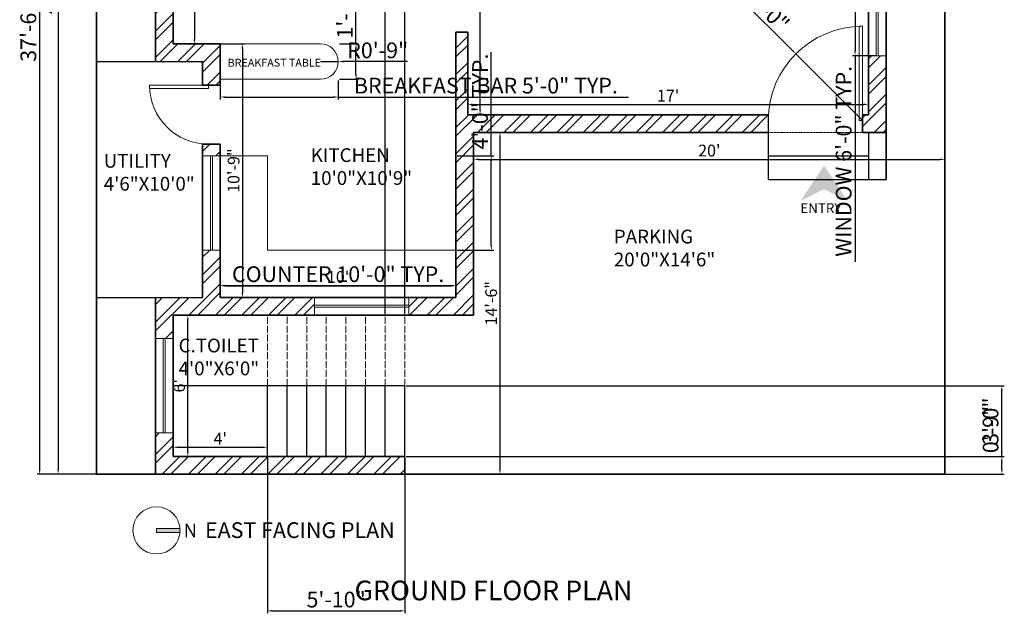
# Model space of a CAD drawing. Units: inches. Extents: x 4732 to 5926, y 2665 to 3255.
# Tile 7 of 8: x 5425 to 5926, y 2665 to 2967. Entities that reach past the tile are written whole.
import ezdxf

# ---------------------------------------------------------------- set-up
doc = ezdxf.new("R2010")
doc.units = ezdxf.units.IN
doc.linetypes.add('ACAD_ISO02W100', pattern=[15, 12, -3])
for name, color, linetype, lineweight in [('A-ANNO-DIMS', 2, 'Continuous', 18), ('A-ANNO-SYMB', 7, 'Continuous', 18), ('A-ANNO-TEXT', 7, 'Continuous', 18), ('A-ANNO-TITL', 7, 'Continuous', 25), ('A-AREA-IDEN', 7, 'Continuous', 18), ('A-DOOR', 3, 'Continuous', 18), ('A-FLOR', 7, 'Continuous', 25), ('A-FLOR-CASE', 7, 'Continuous', 18), ('A-FLOR-STRS', 7, 'Continuous', 25), ('A-FLOR-STRS-HIDN', 8, 'ACAD_ISO02W100', 18), ('A-GLAZ', 4, 'Continuous', 18), ('A-WALL', 7, 'Continuous', 35), ('A-WALL-PATT', 8, 'Continuous', 13), ('C-PROP', 7, 'Continuous', 35)]:
    doc.layers.add(name, color=color, linetype=linetype, lineweight=lineweight)
doc.styles.get("Standard").update_dxf_attribs({"font": 'arial.ttf'})
doc.dimstyles.new('ISO-25', dxfattribs={"dimtxt": 8, "dimasz": 2.5, "dimexe": 1.25, "dimexo": 0.625, "dimtad": 1, "dimdec": 1, "dimlunit": 3, "dimtxsty": 'Standard', "dimcen": 2.5, "dimadec": 0, "dimazin": 0, "dimtfac": 1, "dimtdec": 1, "dimtmove": 0, "dimatfit": 3, "dimfxl": 1, "dimarcsym": 0})

# ---------------------------------------------------------------- blocks, each defined once
blk = doc.blocks.new('*U19')
for p, q in [((0, 0), (0, -6)), ((30, 0), (30, -6))]:
    blk.add_line(p, q)
blk.add_lwpolyline([(0, 0), (0, 30), (1.75, 30), (1.75, 0)], close=True)
blk.add_arc((0, 0), 30, 0, 90)
blk = doc.blocks.new('*D30')
at = {"layer": 'A-ANNO-DIMS', "color": 0, "lineweight": -2, "transparency": 16777216}
for p, q in [((5463.31, 3215.93), (5443.14, 3215.93)), ((5444.39, 3213.43), (5444.39, 2738.43)), ((5463.31, 2735.93), (5443.14, 2735.93))]:
    blk.add_line(p, q, dxfattribs=at)
at = {"layer": 'A-ANNO-DIMS', "color": 0, "transparency": 16777216}
for points in [[(5443.98, 3213.43), (5444.81, 3213.43), (5444.39, 3215.93)], [(5443.98, 2738.43), (5444.81, 2738.43), (5444.39, 2735.93)]]:
    blk.add_solid(points, dxfattribs=at)
at = {"layer": 'Defpoints', "color": 0, "transparency": 16777216}
for p in [(5463.94, 3215.93), (5444.39, 2735.93), (5463.94, 2735.93)]:
    blk.add_point(p, dxfattribs=at)
at = {"layer": 'A-ANNO-DIMS', "color": 0, "transparency": 16777216, "insert": (5440.71, 2975.93), "char_height": 6, "attachment_point": 5, "rotation": 90}
blk.add_mtext("40'", dxfattribs=at)
blk = doc.blocks.new('*D31')
at = {"layer": 'A-ANNO-DIMS', "color": 0, "lineweight": -2, "transparency": 16777216}
for p, q in [((5502.94, 2750.26), (5502.94, 2750.89)), ((5505.44, 2749.64), (5548.44, 2749.64)), ((5550.94, 2750.26), (5550.94, 2750.89))]:
    blk.add_line(p, q, dxfattribs=at)
at = {"layer": 'A-ANNO-DIMS', "color": 0, "transparency": 16777216}
for points in [[(5505.44, 2750.05), (5505.44, 2749.22), (5502.94, 2749.64)], [(5548.44, 2750.05), (5548.44, 2749.22), (5550.94, 2749.64)]]:
    blk.add_solid(points, dxfattribs=at)
at = {"layer": 'Defpoints', "color": 0, "transparency": 16777216}
for p in [(5502.94, 2749.64), (5550.94, 2749.64), (5550.94, 2749.64)]:
    blk.add_point(p, dxfattribs=at)
at = {"layer": 'A-ANNO-DIMS', "color": 0, "transparency": 16777216, "insert": (5526.94, 2753.26), "char_height": 6, "attachment_point": 5}
blk.add_mtext("4'", dxfattribs=at)
blk = doc.blocks.new('*D32')
at = {"layer": 'A-ANNO-DIMS', "color": 0, "lineweight": -2, "transparency": 16777216}
for p, q in [((5503.56, 2816.93), (5511.66, 2816.93)), ((5510.41, 2747.43), (5510.41, 2814.43)), ((5503.56, 2744.93), (5511.66, 2744.93))]:
    blk.add_line(p, q, dxfattribs=at)
at = {"layer": 'A-ANNO-DIMS', "color": 0, "transparency": 16777216}
for points in [[(5510, 2814.43), (5510.83, 2814.43), (5510.41, 2816.93)], [(5510, 2747.43), (5510.83, 2747.43), (5510.41, 2744.93)]]:
    blk.add_solid(points, dxfattribs=at)
at = {"layer": 'Defpoints', "color": 0, "transparency": 16777216}
for p in [(5502.94, 2816.93), (5510.41, 2816.93), (5502.94, 2744.93)]:
    blk.add_point(p, dxfattribs=at)
at = {"layer": 'A-ANNO-DIMS', "color": 0, "transparency": 16777216, "insert": (5506.72, 2780.93), "char_height": 6, "attachment_point": 5, "rotation": 90}
blk.add_mtext("6'", dxfattribs=at)
blk = doc.blocks.new('*D33')
at = {"layer": 'A-ANNO-DIMS', "color": 0, "lineweight": -2, "transparency": 16777216}
for p, q in [((5526.94, 2826.56), (5526.94, 2833.08)), ((5646.94, 2826.56), (5646.94, 2833.08)), ((5529.44, 2831.83), (5644.44, 2831.83))]:
    blk.add_line(p, q, dxfattribs=at)
at = {"layer": 'A-ANNO-DIMS', "color": 0, "transparency": 16777216}
for points in [[(5529.44, 2832.25), (5529.44, 2831.42), (5526.94, 2831.83)], [(5644.44, 2832.25), (5644.44, 2831.42), (5646.94, 2831.83)]]:
    blk.add_solid(points, dxfattribs=at)
at = {"layer": 'Defpoints', "color": 0, "transparency": 16777216}
for p in [(5646.94, 2831.83), (5526.94, 2825.93), (5646.94, 2825.93)]:
    blk.add_point(p, dxfattribs=at)
at = {"layer": 'A-ANNO-DIMS', "color": 0, "transparency": 16777216, "insert": (5586.94, 2835.52), "char_height": 6, "attachment_point": 5}
blk.add_mtext("10'", dxfattribs=at)
blk = doc.blocks.new('*D34')
at = {"layer": 'A-ANNO-DIMS', "color": 0, "lineweight": -2, "transparency": 16777216}
for p, q in [((5518.56, 2954.93), (5539.45, 2954.93)), ((5538.2, 2952.43), (5538.2, 2828.43)), ((5527.56, 2825.93), (5539.45, 2825.93))]:
    blk.add_line(p, q, dxfattribs=at)
at = {"layer": 'A-ANNO-DIMS', "color": 0, "transparency": 16777216}
for points in [[(5537.78, 2952.43), (5538.61, 2952.43), (5538.2, 2954.93)], [(5537.78, 2828.43), (5538.61, 2828.43), (5538.2, 2825.93)]]:
    blk.add_solid(points, dxfattribs=at)
at = {"layer": 'Defpoints', "color": 0, "transparency": 16777216}
for p in [(5517.94, 2954.93), (5526.94, 2825.93), (5538.2, 2825.93)]:
    blk.add_point(p, dxfattribs=at)
at = {"layer": 'A-ANNO-DIMS', "color": 0, "transparency": 16777216, "insert": (5534.51, 2890.43), "char_height": 6, "attachment_point": 5, "rotation": 90}
blk.add_mtext('10\'-9"', dxfattribs=at)
blk = doc.blocks.new('*D35')
at = {"layer": 'A-ANNO-DIMS', "color": 0, "lineweight": -2, "transparency": 16777216}
for p, q in [((5503.56, 3050.93), (5515.02, 3050.93)), ((5513.77, 3048.43), (5513.77, 2957.43)), ((5503.56, 2954.93), (5515.02, 2954.93))]:
    blk.add_line(p, q, dxfattribs=at)
at = {"layer": 'A-ANNO-DIMS', "color": 0, "transparency": 16777216}
for points in [[(5513.36, 3048.43), (5514.19, 3048.43), (5513.77, 3050.93)], [(5513.36, 2957.43), (5514.19, 2957.43), (5513.77, 2954.93)]]:
    blk.add_solid(points, dxfattribs=at)
at = {"layer": 'Defpoints', "color": 0, "transparency": 16777216}
for p in [(5502.94, 3050.93), (5502.94, 2954.93), (5513.77, 2954.93)]:
    blk.add_point(p, dxfattribs=at)
at = {"layer": 'A-ANNO-DIMS', "color": 0, "transparency": 16777216, "insert": (5510.08, 3002.93), "char_height": 6, "attachment_point": 5, "rotation": 90}
blk.add_mtext("8'", dxfattribs=at)
blk = doc.blocks.new('*D37')
at = {"layer": 'A-ANNO-DIMS', "color": 0, "lineweight": -2, "transparency": 16777216}
for p, q in [((5652.94, 2919.56), (5652.94, 2925.42)), ((5655.44, 2924.17), (5854.44, 2924.17)), ((5856.94, 2919.56), (5856.94, 2925.42))]:
    blk.add_line(p, q, dxfattribs=at)
at = {"layer": 'A-ANNO-DIMS', "color": 0, "transparency": 16777216}
for points in [[(5655.44, 2924.59), (5655.44, 2923.75), (5652.94, 2924.17)], [(5854.44, 2924.59), (5854.44, 2923.75), (5856.94, 2924.17)]]:
    blk.add_solid(points, dxfattribs=at)
at = {"layer": 'Defpoints', "color": 0, "transparency": 16777216}
for p in [(5856.94, 2924.17), (5652.94, 2918.93), (5856.94, 2918.93)]:
    blk.add_point(p, dxfattribs=at)
at = {"layer": 'A-ANNO-DIMS', "color": 0, "transparency": 16777216, "insert": (5754.94, 2927.81), "char_height": 6, "attachment_point": 5}
blk.add_mtext("17'", dxfattribs=at)
blk = doc.blocks.new('*D38')
at = {"layer": 'A-ANNO-DIMS', "color": 0, "lineweight": -2, "transparency": 16777216}
for p, q in [((5653.56, 3050.93), (5660.5, 3050.93)), ((5659.25, 2921.43), (5659.25, 3048.43)), ((5653.56, 2918.93), (5660.5, 2918.93))]:
    blk.add_line(p, q, dxfattribs=at)
at = {"layer": 'A-ANNO-DIMS', "color": 0, "transparency": 16777216}
for points in [[(5658.83, 3048.43), (5659.67, 3048.43), (5659.25, 3050.93)], [(5658.83, 2921.43), (5659.67, 2921.43), (5659.25, 2918.93)]]:
    blk.add_solid(points, dxfattribs=at)
at = {"layer": 'Defpoints', "color": 0, "transparency": 16777216}
for p in [(5652.94, 3050.93), (5659.25, 3050.93), (5652.94, 2918.93)]:
    blk.add_point(p, dxfattribs=at)
at = {"layer": 'A-ANNO-DIMS', "color": 0, "transparency": 16777216, "insert": (5655.61, 2984.93), "char_height": 6, "attachment_point": 5, "rotation": 90}
blk.add_mtext("11'", dxfattribs=at)
blk = doc.blocks.new('*D52')
at = {"layer": 'A-ANNO-DIMS', "color": 0, "lineweight": -2, "transparency": 16777216}
for p, q in [((5655.94, 2909.31), (5655.94, 2894.94)), ((5895.94, 2909.31), (5895.94, 2894.94)), ((5658.44, 2896.19), (5893.44, 2896.19))]:
    blk.add_line(p, q, dxfattribs=at)
at = {"layer": 'A-ANNO-DIMS', "color": 0, "transparency": 16777216}
for points in [[(5658.44, 2896.61), (5658.44, 2895.78), (5655.94, 2896.19)], [(5893.44, 2896.61), (5893.44, 2895.78), (5895.94, 2896.19)]]:
    blk.add_solid(points, dxfattribs=at)
at = {"layer": 'Defpoints', "color": 0, "transparency": 16777216}
for p in [(5655.94, 2909.93), (5895.94, 2909.93), (5895.94, 2896.19)]:
    blk.add_point(p, dxfattribs=at)
at = {"layer": 'A-ANNO-DIMS', "color": 0, "transparency": 16777216, "insert": (5775.94, 2899.88), "char_height": 6, "attachment_point": 5}
blk.add_mtext("20'", dxfattribs=at)
blk = doc.blocks.new('*D53')
at = {"layer": 'A-ANNO-DIMS', "color": 0, "lineweight": -2, "transparency": 16777216}
for p, q in [((5656.56, 2909.93), (5670.58, 2909.93)), ((5669.33, 2907.43), (5669.33, 2738.43)), ((5656.56, 2735.93), (5670.58, 2735.93))]:
    blk.add_line(p, q, dxfattribs=at)
at = {"layer": 'A-ANNO-DIMS', "color": 0, "transparency": 16777216}
for points in [[(5668.92, 2907.43), (5669.75, 2907.43), (5669.33, 2909.93)], [(5668.92, 2738.43), (5669.75, 2738.43), (5669.33, 2735.93)]]:
    blk.add_solid(points, dxfattribs=at)
at = {"layer": 'Defpoints', "color": 0, "transparency": 16777216}
for p in [(5655.94, 2909.93), (5655.94, 2735.93), (5669.33, 2735.93)]:
    blk.add_point(p, dxfattribs=at)
at = {"layer": 'A-ANNO-DIMS', "color": 0, "transparency": 16777216, "insert": (5665.64, 2822.93), "char_height": 6, "attachment_point": 5, "rotation": 90}
blk.add_mtext('14\'-6"', dxfattribs=at)
blk = doc.blocks.new('GLAZ-UNIT-48IN')
for p, q in [((0, 1), (48, 1)), ((0, 0), (48, 0))]:
    blk.add_line(p, q)
blk = doc.blocks.new('GLAZ-UNIT-72IN')
for p, q in [((0, 72), (0, 0)), ((1, 72), (1, 0))]:
    blk.add_line(p, q)
blk = doc.blocks.new('COUNTER-KITCHEN-L')
for p, q in [((0, 48), (24, 48)), ((24, 0), (24, 48)), ((24, 0), (120, 0))]:
    blk.add_line(p, q)
blk = doc.blocks.new('COUNTER-BREAKFAST')
for p, q in [((0, 18), (51.1, 18)), ((0, 0), (51.1, 0))]:
    blk.add_line(p, q)
blk.add_arc((51.1, 9), 9, 270, 90)
blk = doc.blocks.new('NORTH-INDICATOR')
at = {"transparency": 33554687}
h = blk.add_hatch(color=256, dxfattribs=at)
h.dxf.hatch_style = 1
h.paths.add_polyline_path([(0, 1), (0, -1), (11.96, -1, 0.020861), (12, 0, 0.020861), (11.96, 1)])
for p, q in [((0, -1), (0, 1)), ((0, 1), (11.96, 1)), ((12, -1), (0, -1))]:
    blk.add_line(p, q)
blk.add_circle((0, 0), 12)
blk.add_text('N', height=6.9).set_placement((13.83, -3.53))
blk = doc.blocks.new('*D68')
at = {"layer": 'A-ANNO-DIMS', "color": 0, "lineweight": -2, "transparency": 16777216}
for p, q in [((5860.31, 3020.93), (5848.89, 3020.93)), ((5850.14, 3018.43), (5850.14, 2951.43)), ((5860.31, 2948.93), (5848.89, 2948.93)), ((5850.14, 2948.93), (5850.14, 2843.95))]:
    blk.add_line(p, q, dxfattribs=at)
at = {"layer": 'A-ANNO-DIMS', "color": 0, "transparency": 16777216}
for points in [[(5849.72, 3018.43), (5850.55, 3018.43), (5850.14, 3020.93)], [(5849.72, 2951.43), (5850.55, 2951.43), (5850.14, 2948.93)]]:
    blk.add_solid(points, dxfattribs=at)
at = {"layer": 'Defpoints', "color": 0, "transparency": 16777216}
for p in [(5860.94, 3020.93), (5850.14, 2948.93), (5860.94, 2948.93)]:
    blk.add_point(p, dxfattribs=at)
at = {"layer": 'A-ANNO-DIMS', "color": 0, "transparency": 16777216, "insert": (5845.37, 2895.19), "char_height": 8, "attachment_point": 5, "rotation": 90}
blk.add_mtext('WINDOW 6\'-0" TYP.', dxfattribs=at)
blk = doc.blocks.new('*D70')
at = {"layer": 'A-ANNO-DIMS', "color": 0, "lineweight": -2, "transparency": 16777216}
for p, q in [((5526.94, 2849.31), (5526.94, 2830.68)), ((5646.94, 2849.31), (5646.94, 2830.68)), ((5529.44, 2831.93), (5644.44, 2831.93))]:
    blk.add_line(p, q, dxfattribs=at)
at = {"layer": 'A-ANNO-DIMS', "color": 0, "transparency": 16777216}
for points in [[(5529.44, 2832.35), (5529.44, 2831.52), (5526.94, 2831.93)], [(5644.44, 2832.35), (5644.44, 2831.52), (5646.94, 2831.93)]]:
    blk.add_solid(points, dxfattribs=at)
at = {"layer": 'Defpoints', "color": 0, "transparency": 16777216}
for p in [(5526.94, 2849.93), (5646.94, 2849.93), (5646.94, 2831.93)]:
    blk.add_point(p, dxfattribs=at)
at = {"layer": 'A-ANNO-DIMS', "color": 0, "transparency": 16777216, "insert": (5586.94, 2836.7), "char_height": 8, "attachment_point": 5}
blk.add_mtext('COUNTER 10\'-0" TYP.', dxfattribs=at)
blk = doc.blocks.new('*D71')
at = {"layer": 'A-ANNO-DIMS', "color": 0, "lineweight": -2, "transparency": 16777216}
for p, q in [((5664.94, 2897.93), (5664.94, 2950.77)), ((5647.56, 2897.93), (5666.19, 2897.93)), ((5664.94, 2852.43), (5664.94, 2895.43)), ((5647.56, 2849.93), (5666.19, 2849.93))]:
    blk.add_line(p, q, dxfattribs=at)
at = {"layer": 'A-ANNO-DIMS', "color": 0, "transparency": 16777216}
for points in [[(5664.52, 2895.43), (5665.35, 2895.43), (5664.94, 2897.93)], [(5664.52, 2852.43), (5665.35, 2852.43), (5664.94, 2849.93)]]:
    blk.add_solid(points, dxfattribs=at)
at = {"layer": 'Defpoints', "color": 0, "transparency": 16777216}
for p in [(5646.94, 2897.93), (5664.94, 2897.93), (5646.94, 2849.93)]:
    blk.add_point(p, dxfattribs=at)
at = {"layer": 'A-ANNO-DIMS', "color": 0, "transparency": 16777216, "insert": (5660.23, 2925.6), "char_height": 8, "attachment_point": 5, "rotation": 90}
blk.add_mtext('4\'-0" TYP.', dxfattribs=at)
blk = doc.blocks.new('*D72')
at = {"layer": 'A-ANNO-DIMS', "color": 0, "lineweight": -2, "transparency": 16777216}
for p, q in [((5526.94, 2936.31), (5526.94, 2926.67)), ((5587.04, 2936.31), (5587.04, 2926.67)), ((5529.44, 2927.92), (5584.54, 2927.92)), ((5587.04, 2927.92), (5734.84, 2927.92))]:
    blk.add_line(p, q, dxfattribs=at)
at = {"layer": 'A-ANNO-DIMS', "color": 0, "transparency": 16777216}
for points in [[(5529.44, 2928.33), (5529.44, 2927.5), (5526.94, 2927.92)], [(5584.54, 2928.33), (5584.54, 2927.5), (5587.04, 2927.92)]]:
    blk.add_solid(points, dxfattribs=at)
at = {"layer": 'Defpoints', "color": 0, "transparency": 16777216}
for p in [(5526.94, 2936.93), (5587.04, 2936.93), (5587.04, 2927.92)]:
    blk.add_point(p, dxfattribs=at)
at = {"layer": 'A-ANNO-DIMS', "color": 0, "transparency": 16777216, "insert": (5662.19, 2932.68), "char_height": 8, "attachment_point": 5}
blk.add_mtext('BREAKFAST BAR 5\'-0" TYP.', dxfattribs=at)
blk = doc.blocks.new('*D73')
at = {"layer": 'A-ANNO-DIMS', "color": 0, "lineweight": -2, "transparency": 16777216}
for p, q in [((5596.05, 2954.93), (5596.05, 3006.69)), ((5587.66, 2954.93), (5597.3, 2954.93)), ((5596.05, 2939.43), (5596.05, 2952.43)), ((5587.66, 2936.93), (5597.3, 2936.93))]:
    blk.add_line(p, q, dxfattribs=at)
at = {"layer": 'A-ANNO-DIMS', "color": 0, "transparency": 16777216}
for points in [[(5595.64, 2952.43), (5596.47, 2952.43), (5596.05, 2954.93)], [(5595.64, 2939.43), (5596.47, 2939.43), (5596.05, 2936.93)]]:
    blk.add_solid(points, dxfattribs=at)
at = {"layer": 'Defpoints', "color": 0, "transparency": 16777216}
for p in [(5587.04, 2954.93), (5596.05, 2954.93), (5587.04, 2936.93)]:
    blk.add_point(p, dxfattribs=at)
at = {"layer": 'A-ANNO-DIMS', "color": 0, "transparency": 16777216, "insert": (5591.34, 2982.06), "char_height": 8, "attachment_point": 5, "rotation": 90}
blk.add_mtext('1\'-6" TYP.', dxfattribs=at)
blk = doc.blocks.new('*D105')
at = {"layer": 'A-ANNO-DIMS', "color": 0, "lineweight": -2, "transparency": 16777216}
for p, q in [((5493.31, 3185.93), (5433.74, 3185.93)), ((5434.99, 3183.43), (5434.99, 2738.43)), ((5493.31, 2735.93), (5433.74, 2735.93))]:
    blk.add_line(p, q, dxfattribs=at)
at = {"layer": 'A-ANNO-DIMS', "color": 0, "transparency": 16777216}
for points in [[(5434.57, 3183.43), (5435.4, 3183.43), (5434.99, 3185.93)], [(5434.57, 2738.43), (5435.4, 2738.43), (5434.99, 2735.93)]]:
    blk.add_solid(points, dxfattribs=at)
at = {"layer": 'Defpoints', "color": 0, "transparency": 16777216}
for p in [(5493.94, 3185.93), (5434.99, 2735.93), (5493.94, 2735.93)]:
    blk.add_point(p, dxfattribs=at)
at = {"layer": 'A-ANNO-DIMS', "color": 0, "transparency": 16777216, "insert": (5430.27, 2960.93), "char_height": 8, "attachment_point": 5, "rotation": 90}
blk.add_mtext('37\'-6"', dxfattribs=at)
blk = doc.blocks.new('*D110')
at = {"layer": 'A-ANNO-DIMS', "color": 0, "lineweight": -2, "transparency": 16777216}
for p, q in [((5550.94, 2744.31), (5550.94, 2665.12)), ((5620.94, 2744.31), (5620.94, 2665.12)), ((5553.44, 2666.37), (5618.44, 2666.37))]:
    blk.add_line(p, q, dxfattribs=at)
at = {"layer": 'A-ANNO-DIMS', "color": 0, "transparency": 16777216}
for points in [[(5553.44, 2666.79), (5553.44, 2665.96), (5550.94, 2666.37)], [(5618.44, 2666.79), (5618.44, 2665.96), (5620.94, 2666.37)]]:
    blk.add_solid(points, dxfattribs=at)
at = {"layer": 'Defpoints', "color": 0, "transparency": 16777216}
for p in [(5550.94, 2744.93), (5620.94, 2744.93), (5620.94, 2666.37)]:
    blk.add_point(p, dxfattribs=at)
at = {"layer": 'A-ANNO-DIMS', "color": 0, "transparency": 16777216, "insert": (5585.94, 2671.08), "char_height": 8, "attachment_point": 5}
blk.add_mtext('5\'-10"', dxfattribs=at)
blk = doc.blocks.new('*D111')
at = {"layer": 'A-ANNO-DIMS', "color": 0, "lineweight": -2, "transparency": 16777216}
for p, q in [((5610.94, 2817.56), (5610.94, 3246.13)), ((5613.44, 3244.88), (5618.44, 3244.88)), ((5620.94, 2817.56), (5620.94, 3246.13)), ((5620.94, 3244.88), (5652.17, 3244.88))]:
    blk.add_line(p, q, dxfattribs=at)
at = {"layer": 'A-ANNO-DIMS', "color": 0, "transparency": 16777216}
for points in [[(5613.44, 3245.3), (5613.44, 3244.47), (5610.94, 3244.88)], [(5618.44, 3245.3), (5618.44, 3244.47), (5620.94, 3244.88)]]:
    blk.add_solid(points, dxfattribs=at)
at = {"layer": 'Defpoints', "color": 0, "transparency": 16777216}
for p in [(5620.94, 3244.88), (5610.94, 2816.93), (5620.94, 2816.93)]:
    blk.add_point(p, dxfattribs=at)
at = {"layer": 'A-ANNO-DIMS', "color": 0, "transparency": 16777216, "insert": (5637.8, 3249.59), "char_height": 8, "attachment_point": 5}
blk.add_mtext('0\'-10"', dxfattribs=at)
blk = doc.blocks.new('*D112')
at = {"layer": 'A-ANNO-DIMS', "color": 0, "lineweight": -2, "transparency": 16777216}
for p, q in [((5621.56, 2780.93), (5926.14, 2780.93)), ((5924.89, 2747.43), (5924.89, 2778.43)), ((5621.56, 2744.93), (5926.14, 2744.93))]:
    blk.add_line(p, q, dxfattribs=at)
at = {"layer": 'A-ANNO-DIMS', "color": 0, "transparency": 16777216}
for points in [[(5924.47, 2778.43), (5925.3, 2778.43), (5924.89, 2780.93)], [(5924.47, 2747.43), (5925.3, 2747.43), (5924.89, 2744.93)]]:
    blk.add_solid(points, dxfattribs=at)
at = {"layer": 'Defpoints', "color": 0, "transparency": 16777216}
for p in [(5620.94, 2780.93), (5924.89, 2780.93), (5620.94, 2744.93)]:
    blk.add_point(p, dxfattribs=at)
at = {"layer": 'A-ANNO-DIMS', "color": 0, "transparency": 16777216, "insert": (5920.17, 2762.93), "char_height": 8, "attachment_point": 5, "rotation": 90}
blk.add_mtext('3\'-0"', dxfattribs=at)
blk = doc.blocks.new('*D113')
at = {"layer": 'A-ANNO-DIMS', "color": 0, "lineweight": -2, "transparency": 16777216}
for p, q in [((5924.89, 2744.93), (5924.89, 2769.95)), ((5621.56, 2744.93), (5926.14, 2744.93)), ((5924.89, 2738.43), (5924.89, 2742.43)), ((5621.56, 2735.93), (5926.14, 2735.93))]:
    blk.add_line(p, q, dxfattribs=at)
at = {"layer": 'A-ANNO-DIMS', "color": 0, "transparency": 16777216}
for points in [[(5924.47, 2742.43), (5925.3, 2742.43), (5924.89, 2744.93)], [(5924.47, 2738.43), (5925.3, 2738.43), (5924.89, 2735.93)]]:
    blk.add_solid(points, dxfattribs=at)
at = {"layer": 'Defpoints', "color": 0, "transparency": 16777216}
for p in [(5620.94, 2744.93), (5924.89, 2744.93), (5620.94, 2735.93)]:
    blk.add_point(p, dxfattribs=at)
at = {"layer": 'A-ANNO-DIMS', "color": 0, "transparency": 16777216, "insert": (5920.18, 2758.69), "char_height": 8, "attachment_point": 5, "rotation": 90}
blk.add_mtext('0\'-9"', dxfattribs=at)
blk = doc.blocks.new('*D117')
at = {"layer": 'A-ANNO-DIMS', "color": 0, "lineweight": -2, "transparency": 16777216}
for p, q in [((5788.96, 2980.91), (5818.23, 2951.64)), ((5853.94, 2915.93), (5820, 2949.87))]:
    blk.add_line(p, q, dxfattribs=at)
at = {"layer": 'A-ANNO-DIMS', "color": 0, "transparency": 16777216}
blk.add_solid([(5818.52, 2951.94), (5817.93, 2951.35), (5820, 2949.87)], dxfattribs=at)
at = {"layer": 'Defpoints', "color": 0, "transparency": 16777216}
for p in [(5820, 2949.87), (5853.94, 2915.93)]:
    blk.add_point(p, dxfattribs=at)
at = {"layer": 'A-ANNO-DIMS', "color": 0, "transparency": 16777216, "insert": (5802.96, 2973.57), "char_height": 8, "attachment_point": 5, "rotation": 315.0001}
blk.add_mtext('R4\'-0"', dxfattribs=at)
blk = doc.blocks.new('*D118')
at = {"layer": 'A-ANNO-DIMS', "color": 0, "lineweight": -2, "transparency": 16777216}
for p, q in [((5578.04, 2945.93), (5587.04, 2945.93)), ((5622.21, 2945.93), (5589.54, 2945.93))]:
    blk.add_line(p, q, dxfattribs=at)
at = {"layer": 'A-ANNO-DIMS', "color": 0, "transparency": 16777216}
blk.add_solid([(5589.54, 2946.35), (5589.54, 2945.52), (5587.04, 2945.93)], dxfattribs=at)
at = {"layer": 'Defpoints', "color": 0, "transparency": 16777216}
for p in [(5578.04, 2945.93), (5587.04, 2945.93)]:
    blk.add_point(p, dxfattribs=at)
at = {"layer": 'A-ANNO-DIMS', "color": 0, "transparency": 16777216, "insert": (5607.12, 2950.64), "char_height": 8, "attachment_point": 5, "rotation": 359.9979}
blk.add_mtext('R0\'-9"', dxfattribs=at)

msp = doc.modelspace()

# ---------------------------------------------------------------- hatches: boundary and pattern name
at = {"layer": 'A-ANNO-SYMB'}
h = msp.add_hatch(color=256, dxfattribs=at)
h.dxf.hatch_style = 1
h.paths.add_polyline_path([(5834.34, 2881.01), (5846.34, 2875.01), (5834.34, 2893.01), (5822.34, 2875.01)])
at = {"layer": 'A-WALL-PATT'}
h = msp.add_hatch(dxfattribs=at)
h.set_pattern_fill('ANSI32', color=256)
h.paths.add_polyline_path([(5502.94, 3086.93), (5493.94, 3086.93), (5493.94, 3026.93), (5502.94, 3026.93), (5502.94, 3050.93), (5646.94, 3050.93), (5646.94, 3008.93), (5652.94, 3008.93), (5652.94, 3050.93), (5667.94, 3050.93), (5667.94, 3056.93), (5502.94, 3056.93)])
h.paths.add_polyline_path([(5502.94, 2978.93), (5493.94, 2978.93), (5493.94, 2945.93), (5517.94, 2945.93), (5517.94, 2933.93), (5520.94, 2933.93), (5526.94, 2933.93), (5526.94, 2954.93), (5502.94, 2954.93)])
h.paths.add_polyline_path([(5526.94, 2849.93), (5517.94, 2849.93), (5517.94, 2825.93), (5493.94, 2825.93), (5493.94, 2804.93), (5502.94, 2804.93), (5502.94, 2816.93), (5574.94, 2816.93), (5574.94, 2825.93), (5526.94, 2825.93)])
h.paths.add_polyline_path([(5526.94, 2903.93), (5520.94, 2903.93), (5517.94, 2903.93), (5517.94, 2897.93), (5526.94, 2897.93)])
h.paths.add_polyline_path([(5655.94, 2909.93), (5805.94, 2909.93), (5805.94, 2915.93), (5805.94, 2918.93), (5652.94, 2918.93), (5652.94, 2960.93), (5646.94, 2960.93), (5646.94, 2825.93), (5622.94, 2825.93), (5622.94, 2816.93), (5655.94, 2816.93)])
h.paths.add_polyline_path([(5620.94, 2744.93), (5502.94, 2744.93), (5502.94, 2756.93), (5493.94, 2756.93), (5493.94, 2735.93), (5620.94, 2735.93)])
h.paths.add_polyline_path([(5865.94, 2948.93), (5856.94, 2948.93), (5856.94, 2918.93), (5853.94, 2918.93), (5853.94, 2915.93), (5853.94, 2909.93), (5865.94, 2909.93)])
h.paths.add_polyline_path([(5865.94, 3086.93), (5856.94, 3086.93), (5856.94, 3056.93), (5751.94, 3056.93), (5751.94, 3050.93), (5856.94, 3050.93), (5856.94, 3020.93), (5865.94, 3020.93)])
h.paths.add_polyline_path([(5865.94, 3185.93), (5808.94, 3185.93), (5808.94, 3176.93), (5856.94, 3176.93), (5856.94, 3146.93), (5865.94, 3146.93)])
h.paths.add_polyline_path([(5760.94, 3185.93), (5691.94, 3185.93), (5691.94, 3176.93), (5706.94, 3176.93), (5706.94, 3104.93), (5703.94, 3104.93), (5703.94, 3098.93), (5706.94, 3098.93), (5706.94, 3056.93), (5703.94, 3056.93), (5703.94, 3050.93), (5706.94, 3050.93), (5715.94, 3050.93), (5715.94, 3056.93), (5712.94, 3056.93), (5712.94, 3176.93), (5760.94, 3176.93)])
h.paths.add_polyline_path([(5667.94, 3185.93), (5598.94, 3185.93), (5598.94, 3176.93), (5646.94, 3176.93), (5646.94, 3098.93), (5673.94, 3098.93), (5673.94, 3104.93), (5652.94, 3104.93), (5652.94, 3176.93), (5667.94, 3176.93)])
h.paths.add_polyline_path([(5550.94, 3185.93), (5493.94, 3185.93), (5493.94, 3146.93), (5502.94, 3146.93), (5502.94, 3176.93), (5550.94, 3176.93)])

# ---------------------------------------------------------------- linework, layer by layer
at = {"layer": 'A-DOOR'}
for p, q in [((5805.94, 2915.93), (5805.94, 2909.93)), ((5853.94, 2915.93), (5853.94, 2909.93))]:
    msp.add_line(p, q, dxfattribs=at)
msp.add_lwpolyline([(5853.94, 2915.93), (5853.94, 2963.93), (5852.19, 2963.93), (5852.19, 2915.93)], close=True, dxfattribs=at)
msp.add_arc((5853.94, 2915.93), 48, 90, 180, dxfattribs=at)
at = {"layer": 'A-FLOR'}
for p, q in [((5463.94, 2945.93), (5517.94, 2945.93)), ((5463.94, 2825.93), (5517.94, 2825.93))]:
    msp.add_line(p, q, dxfattribs=at)
at = {"layer": 'A-FLOR-STRS'}
for p, q in [((5805.94, 2918.93), (5805.94, 2885.93)), ((5856.94, 2909.93), (5856.94, 2885.93)), ((5805.94, 2897.93), (5856.94, 2897.93)), ((5805.94, 2885.93), (5865.94, 2885.93)), ((5620.94, 2780.93), (5502.94, 2780.93)), ((5550.94, 2744.93), (5550.94, 2780.93)), ((5560.94, 2744.93), (5560.94, 2780.93)), ((5570.94, 2744.93), (5570.94, 2780.93)), ((5580.94, 2744.93), (5580.94, 2780.93)), ((5590.94, 2744.93), (5590.94, 2780.93)), ((5600.94, 2744.93), (5600.94, 2780.93)), ((5610.94, 2744.93), (5610.94, 2780.93)), ((5620.94, 2735.93), (5620.94, 2780.93))]:
    msp.add_line(p, q, dxfattribs=at)
at = {"layer": 'A-FLOR-STRS-HIDN', "ltscale": 0.1}
msp.add_line((5805.94, 2909.93), (5853.94, 2909.93), dxfattribs=at)
at = {"layer": 'A-FLOR-STRS-HIDN', "ltscale": 0.3}
for p, q in [((5550.94, 2780.93), (5550.94, 2816.93)), ((5560.94, 2780.93), (5560.94, 2816.93)), ((5570.94, 2780.93), (5570.94, 2816.93)), ((5580.94, 2780.93), (5580.94, 2816.93)), ((5590.94, 2780.93), (5590.94, 2816.93)), ((5600.94, 2780.93), (5600.94, 2816.93)), ((5610.94, 2780.93), (5610.94, 2816.93)), ((5620.94, 2780.93), (5620.94, 2816.93))]:
    msp.add_line(p, q, dxfattribs=at)
at = {"layer": 'A-GLAZ'}
for p, q in [((5856.94, 2948.93), (5865.94, 2948.93)), ((5517.94, 2897.93), (5526.94, 2897.93)), ((5517.94, 2849.93), (5526.94, 2849.93)), ((5574.94, 2816.93), (5574.94, 2825.93)), ((5622.94, 2816.93), (5622.94, 2825.93)), ((5502.94, 2804.93), (5493.94, 2804.93)), ((5502.94, 2756.93), (5493.94, 2756.93))]:
    msp.add_line(p, q, dxfattribs=at)
at = {"layer": 'A-WALL'}
for p, q in [((5493.94, 2945.93), (5493.94, 3185.93)), ((5865.94, 3185.93), (5865.94, 2885.93)), ((5502.94, 2954.93), (5502.94, 3050.93)), ((5856.94, 3050.93), (5856.94, 2918.93)), ((5646.94, 2960.93), (5652.94, 2960.93)), ((5646.94, 2825.93), (5646.94, 2960.93)), ((5652.94, 2918.93), (5652.94, 2960.93)), ((5502.94, 2954.93), (5526.94, 2954.93)), ((5526.94, 2933.93), (5526.94, 2954.93)), ((5517.94, 2933.93), (5517.94, 2945.93)), ((5517.94, 2933.93), (5526.94, 2933.93)), ((5652.94, 2918.93), (5805.94, 2918.93)), ((5853.94, 2918.93), (5856.94, 2918.93)), ((5853.94, 2918.93), (5853.94, 2909.93)), ((5655.94, 2909.93), (5805.94, 2909.93)), ((5655.94, 2816.93), (5655.94, 2909.93)), ((5853.94, 2909.93), (5865.94, 2909.93)), ((5517.94, 2825.93), (5517.94, 2903.93)), ((5517.94, 2903.93), (5526.94, 2903.93)), ((5526.94, 2825.93), (5526.94, 2903.93)), ((5493.94, 2735.93), (5493.94, 2825.93)), ((5526.94, 2825.93), (5646.94, 2825.93)), ((5502.94, 2816.93), (5655.94, 2816.93)), ((5502.94, 2744.93), (5502.94, 2816.93)), ((5620.94, 2744.93), (5502.94, 2744.93))]:
    msp.add_line(p, q, dxfattribs=at)
at = {"layer": 'C-PROP'}
msp.add_lwpolyline([(5463.94, 3215.93), (5895.94, 3215.93), (5895.94, 2735.93), (5463.94, 2735.93)], close=True, dxfattribs=at)

# ---------------------------------------------------------------- block references
at = {"layer": 'A-ANNO-SYMB'}
msp.add_blockref('NORTH-INDICATOR', (5494.48, 2707.32), dxfattribs=at)
at = {"layer": 'A-DOOR', "xscale": -1, "rotation": 90}
msp.add_blockref('*U19', (5520.94, 2933.93), dxfattribs=at)
at = {"layer": 'A-FLOR-CASE'}
for name, p in [('COUNTER-BREAKFAST', (5526.94, 2936.93)), ('COUNTER-KITCHEN-L', (5526.94, 2849.93))]:
    msp.add_blockref(name, p, dxfattribs=at)
at = {"layer": 'A-GLAZ'}
for name, p, rotation in [('GLAZ-UNIT-72IN', (5861.94, 3020.93), 180), ('GLAZ-UNIT-48IN', (5521.94, 2897.93), 270), ('GLAZ-UNIT-48IN', (5622.94, 2821.93), 180), ('GLAZ-UNIT-48IN', (5497.94, 2804.93), 270)]:
    msp.add_blockref(name, p, dxfattribs=dict(at, rotation=rotation))

# ---------------------------------------------------------------- texts
at = {"layer": 'A-ANNO-TEXT', "attachment_point": 1}
for s, width, insert, char_height in [('BREAKFAST TABLE', 72.2298, (5530.73, 2947.38), 4), ('{\\fTimes New Roman|b0|i0|c0|p18;ENTRY}', 196.2607, (5822.27, 2873.88), 5)]:
    msp.add_mtext_dynamic_manual_height_columns(s, width=width, gutter_width=12.5, heights=[0], dxfattribs=dict(at, insert=insert, char_height=char_height))
at = {"layer": 'A-ANNO-TITL', "attachment_point": 1}
for s, insert, char_height in [('{\\fTimes New Roman|b0|i0|c0|p18;EAST FACING PLAN}', (5519.18, 2711.44), 8), ('{\\fTimes New Roman|b0|i0|c0|p18;GROUND FLOOR PLAN}', (5595.3, 2681.77), 10)]:
    msp.add_mtext_dynamic_manual_height_columns(s, width=196.2607, gutter_width=12.5, heights=[0], dxfattribs=dict(at, insert=insert, char_height=char_height))
at = {"layer": 'A-AREA-IDEN', "char_height": 7, "attachment_point": 1}
for s, insert in [('{\\fTimes New Roman|b0|i0|c0|p18;UTILITY\\P4\'6"X10\'0"}', (5467.6, 2898.93)), ('{\\fTimes New Roman|b0|i0|c0|p18;KITCHEN\\P10\'0"X10\'9"}', (5573.01, 2901.84)), ('{\\fTimes New Roman|b0|i0|c0|p18;PARKING\\P20\'0"X14\'6"}', (5727.32, 2860.38)), ('{\\fTimes New Roman|b0|i0|c0|p18;C.TOILET\\P4\'0"X6\'0"}', (5505.72, 2804.93))]:
    msp.add_mtext_dynamic_manual_height_columns(s, width=61.0557, gutter_width=12.5, heights=[0], dxfattribs=dict(at, insert=insert))

# ---------------------------------------------------------------- dimensions: what is measured, and where the dimension line sits
at = {"layer": 'A-ANNO-DIMS'}
for base, p1, p2, override, picture, middle in [((5620.94, 3244.88), (5610.94, 2816.93), (5620.94, 2816.93), {"dimdec": 1, "dimlfac": 1, "dimrnd": 0, "dimzin": 1, "dimdsep": 46, "dimlunit": 4, "dimfrac": 2}, '*D111', (5637.8, 3249.59)), ((5856.94, 2924.17), (5652.94, 2918.93), (5856.94, 2918.93), {"dimtxt": 6, "dimclrd": 0, "dimclre": 0, "dimclrt": 0}, '*D37', (5754.94, 2927.81)), ((5895.94, 2896.19), (5655.94, 2909.93), (5895.94, 2909.93), {"dimtxt": 6, "dimclrd": 0, "dimclre": 0, "dimclrt": 0}, '*D52', (5775.94, 2899.88)), ((5646.94, 2831.83), (5526.94, 2825.93), (5646.94, 2825.93), {"dimtxt": 6, "dimclrd": 0, "dimclre": 0, "dimclrt": 0}, '*D33', (5586.94, 2835.52)), ((5550.94, 2749.64), (5502.94, 2749.64), (5550.94, 2749.64), {"dimtxt": 6, "dimclrd": 0, "dimclre": 0, "dimclrt": 0}, '*D31', (5526.94, 2753.26)), ((5620.94, 2666.37), (5550.94, 2744.93), (5620.94, 2744.93), {"dimdec": 1, "dimlfac": 1, "dimrnd": 0, "dimzin": 1, "dimdsep": 46, "dimlunit": 4, "dimfrac": 2}, '*D110', (5585.94, 2671.08))]:
    dim = msp.add_linear_dim(base=base, p1=p1, p2=p2, dimstyle='ISO-25', override=override, dxfattribs=at)
    dim.commit()
    dim.dimension.update_dxf_attribs({"geometry": picture, "text_midpoint": middle})
for base, p1, p2, override, picture, middle in [((5444.39, 2735.93), (5463.94, 3215.93), (5463.94, 2735.93), {"dimtxt": 6, "dimclrd": 0, "dimclre": 0, "dimclrt": 0}, '*D30', (5440.71, 2975.93)), ((5434.99, 2735.93), (5493.94, 3185.93), (5493.94, 2735.93), {"dimdec": 1, "dimlfac": 1, "dimrnd": 0, "dimzin": 1, "dimdsep": 46, "dimlunit": 4, "dimfrac": 2}, '*D105', (5430.27, 2960.93)), ((5513.77, 2954.93), (5502.94, 3050.93), (5502.94, 2954.93), {"dimtxt": 6, "dimclrd": 0, "dimclre": 0, "dimclrt": 0}, '*D35', (5510.08, 3002.93)), ((5659.25, 3050.93), (5652.94, 2918.93), (5652.94, 3050.93), {"dimtxt": 6, "dimclrd": 0, "dimclre": 0, "dimclrt": 0}, '*D38', (5655.61, 2984.93)), ((5538.2, 2825.93), (5517.94, 2954.93), (5526.94, 2825.93), {"dimtxt": 6, "dimclrd": 0, "dimclre": 0, "dimclrt": 0}, '*D34', (5534.51, 2890.43)), ((5669.33, 2735.93), (5655.94, 2909.93), (5655.94, 2735.93), {"dimtxt": 6, "dimclrd": 0, "dimclre": 0, "dimclrt": 0}, '*D53', (5665.64, 2822.93)), ((5510.41, 2816.93), (5502.94, 2744.93), (5502.94, 2816.93), {"dimtxt": 6, "dimclrd": 0, "dimclre": 0, "dimclrt": 0}, '*D32', (5506.72, 2780.93)), ((5924.89, 2780.93), (5620.94, 2744.93), (5620.94, 2780.93), {"dimdec": 1, "dimlfac": 1, "dimrnd": 0, "dimzin": 1, "dimdsep": 46, "dimlunit": 4, "dimfrac": 2}, '*D112', (5920.17, 2762.93)), ((5924.89, 2744.93), (5620.94, 2735.93), (5620.94, 2744.93), {"dimdec": 1, "dimlfac": 1, "dimrnd": 0, "dimzin": 1, "dimdsep": 46, "dimlunit": 4, "dimfrac": 2}, '*D113', (5920.18, 2758.69))]:
    dim = msp.add_linear_dim(base=base, p1=p1, p2=p2, angle=90, dimstyle='ISO-25', override=override, dxfattribs=at)
    dim.commit()
    dim.dimension.update_dxf_attribs({"geometry": picture, "text_midpoint": middle})
for base, p1, p2, angle, text, picture, middle in [((5850.14, 2948.93), (5860.94, 3020.93), (5860.94, 2948.93), 270, 'WINDOW <> TYP.', '*D68', (5845.37, 2895.19)), ((5596.05, 2954.93), (5587.04, 2936.93), (5587.04, 2954.93), 90, '<> TYP.', '*D73', (5591.34, 2982.06)), ((5664.94, 2897.93), (5646.94, 2849.93), (5646.94, 2897.93), 90, '<> TYP.', '*D71', (5660.23, 2925.6))]:
    dim = msp.add_linear_dim(base=base, p1=p1, p2=p2, angle=angle, text=text, dimstyle='ISO-25', override={"dimdec": 1, "dimlfac": 1, "dimrnd": 0, "dimzin": 1, "dimdsep": 46, "dimlunit": 4, "dimfrac": 2}, dxfattribs=at)
    dim.commit()
    dim.dimension.update_dxf_attribs({"geometry": picture, "text_midpoint": middle})
dim = msp.add_radius_dim(center=(5853.94, 2915.93), mpoint=(5820, 2949.87), dimstyle='ISO-25', override={"dimdec": 1, "dimlfac": 1, "dimrnd": 0, "dimzin": 1, "dimdsep": 46, "dimlunit": 4, "dimfrac": 2}, dxfattribs=at)
dim.commit()
dim.dimension.update_dxf_attribs({"geometry": '*D117', "text_midpoint": (5799.63, 2970.24), "dimtype": 164})
for base, p1, p2, text, picture, middle in [((5587.04, 2927.92), (5526.94, 2936.93), (5587.04, 2936.93), 'BREAKFAST BAR <> TYP.', '*D72', (5662.19, 2932.68)), ((5646.94, 2831.93), (5526.94, 2849.93), (5646.94, 2849.93), 'COUNTER <> TYP.', '*D70', (5586.94, 2836.7))]:
    dim = msp.add_linear_dim(base=base, p1=p1, p2=p2, text=text, dimstyle='ISO-25', override={"dimdec": 1, "dimlfac": 1, "dimrnd": 0, "dimzin": 1, "dimdsep": 46, "dimlunit": 4, "dimfrac": 2}, dxfattribs=at)
    dim.commit()
    dim.dimension.update_dxf_attribs({"geometry": picture, "text_midpoint": middle})
dim = msp.add_radius_dim(center=(5578.04, 2945.93), mpoint=(5587.04, 2945.93), dimstyle='ISO-25', override={"dimdec": 1, "dimlfac": 1, "dimrnd": 0, "dimzin": 1, "dimdsep": 46, "dimlunit": 4, "dimfrac": 2}, dxfattribs=at)
dim.commit()
dim.dimension.update_dxf_attribs({"geometry": '*D118', "text_midpoint": (5607.12, 2950.64)})

doc.saveas('drawing.dxf')
